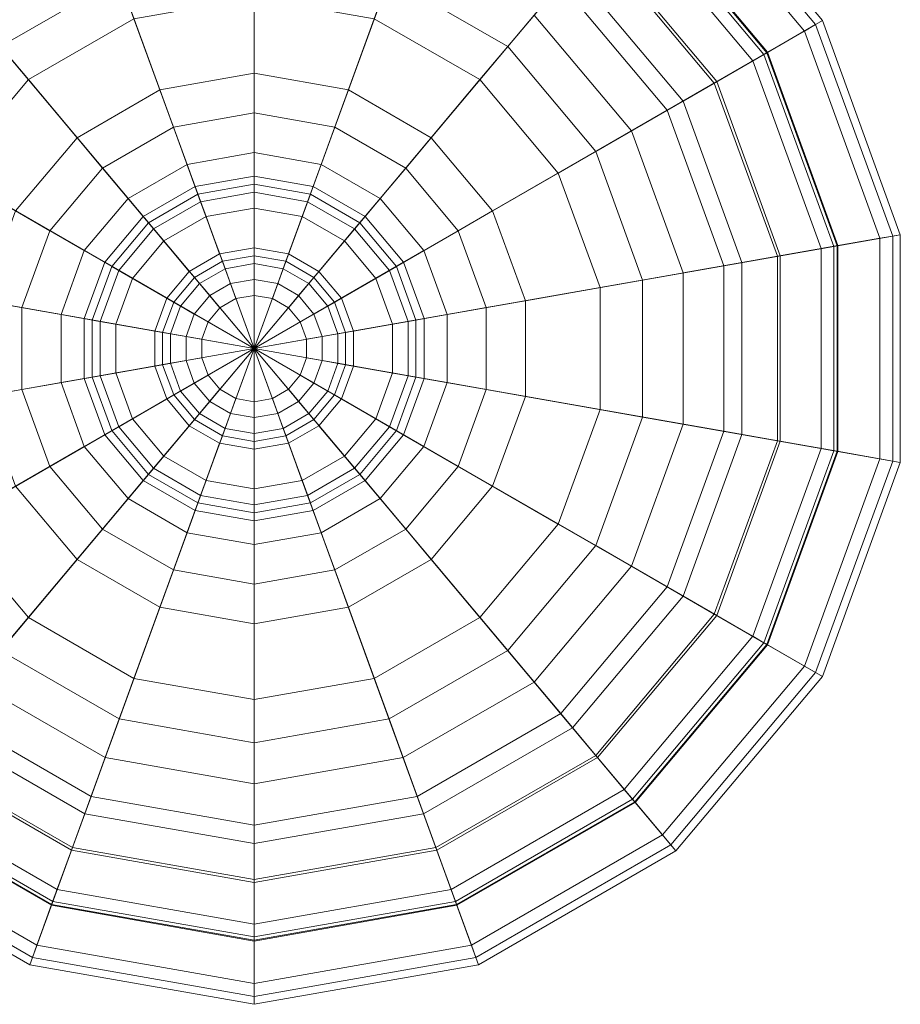
# Model space of a CAD drawing. Units: inches. Extents: x 375 to 1122, y 27 to 1069.
# Tile 14 of 155: x 729.198 to 731.015, y 267.095 to 269.129. Entities that reach past the tile are written whole.
import ezdxf

# ---------------------------------------------------------------- set-up
doc = ezdxf.new("R2010")
doc.units = ezdxf.units.IN
doc.layers.add('Furniture', color=30, linetype='Continuous', lineweight=18)

# ---------------------------------------------------------------- blocks, each defined once
blk = doc.blocks.new('A$C403C54AD')
for points in [[(1.940462, 1.15174, -0.060915), (1.946342, 1.118392, -0.057836), (1.946342, 1.118392, -0.057836), (1.929411, 1.147718, -0.060915)], [(1.941029, 1.148524, -0.057684), (1.940462, 1.15174, -0.060915), (1.929411, 1.147718, -0.060915), (1.931044, 1.144889, -0.057684)], [(1.952223, 1.15174, -0.060915), (1.946342, 1.118392, -0.057836), (1.946342, 1.118392, -0.057836), (1.940462, 1.15174, -0.060915)], [(1.951655, 1.148524, -0.057684), (1.952223, 1.15174, -0.060915), (1.940462, 1.15174, -0.060915), (1.941029, 1.148524, -0.057684)], [(1.963274, 1.147718, -0.060915), (1.946342, 1.118392, -0.057836), (1.946342, 1.118392, -0.057836), (1.952223, 1.15174, -0.060915)], [(1.961641, 1.144889, -0.057684), (1.963274, 1.147718, -0.060915), (1.952223, 1.15174, -0.060915), (1.951655, 1.148524, -0.057684)], [(1.941036, 1.148484, 0.102069), (1.940532, 1.151347, 0.088845), (1.929611, 1.147372, 0.088845), (1.931064, 1.144854, 0.102069)], [(1.940532, 1.151347, 0.088845), (1.940649, 1.150682, 0.060603), (1.929948, 1.146788, 0.060603), (1.929611, 1.147372, 0.088845)], [(1.951648, 1.148484, 0.102069), (1.952153, 1.151347, 0.088845), (1.940532, 1.151347, 0.088845), (1.941036, 1.148484, 0.102069)], [(1.952153, 1.151347, 0.088845), (1.952036, 1.150682, 0.060603), (1.940649, 1.150682, 0.060603), (1.940532, 1.151347, 0.088845)], [(1.96162, 1.144854, 0.102069), (1.963074, 1.147372, 0.088845), (1.952153, 1.151347, 0.088845), (1.951648, 1.148484, 0.102069)], [(1.963074, 1.147372, 0.088845), (1.962737, 1.146788, 0.060603), (1.952036, 1.150682, 0.060603), (1.952153, 1.151347, 0.088845)], [(1.940649, 1.150682, 0.060603), (1.94158, 1.145399, 0.042594), (1.932631, 1.142142, 0.042594), (1.929948, 1.146788, 0.060603)], [(1.952036, 1.150682, 0.060603), (1.951105, 1.145399, 0.042594), (1.94158, 1.145399, 0.042594), (1.940649, 1.150682, 0.060603)], [(1.962737, 1.146788, 0.060603), (1.960054, 1.142142, 0.042594), (1.951105, 1.145399, 0.042594), (1.952036, 1.150682, 0.060603)], [(1.943874, 1.13239, -0.054409), (1.941029, 1.148524, -0.057684), (1.931044, 1.144889, -0.057684), (1.939235, 1.130702, -0.054409)], [(1.941904, 1.143563, 0.111475), (1.941036, 1.148484, 0.102069), (1.931064, 1.144854, 0.102069), (1.933563, 1.140527, 0.111475)], [(1.941067, 1.148309, 0.088628), (1.941555, 1.145542, 0.101264), (1.932558, 1.142268, 0.101264), (1.931153, 1.144701, 0.088628)], [(1.941182, 1.147661, 0.061088), (1.941067, 1.148309, 0.088628), (1.931153, 1.144701, 0.088628), (1.931482, 1.144131, 0.061088)], [(1.948811, 1.13239, -0.054409), (1.951655, 1.148524, -0.057684), (1.941029, 1.148524, -0.057684), (1.943874, 1.13239, -0.054409)], [(1.950781, 1.143563, 0.111475), (1.951648, 1.148484, 0.102069), (1.941036, 1.148484, 0.102069), (1.941904, 1.143563, 0.111475)], [(1.951618, 1.148309, 0.088628), (1.95113, 1.145542, 0.101264), (1.941555, 1.145542, 0.101264), (1.941067, 1.148309, 0.088628)], [(1.951503, 1.147661, 0.061088), (1.951618, 1.148309, 0.088628), (1.941067, 1.148309, 0.088628), (1.941182, 1.147661, 0.061088)], [(1.95345, 1.130702, -0.054409), (1.961641, 1.144889, -0.057684), (1.951655, 1.148524, -0.057684), (1.948811, 1.13239, -0.054409)], [(1.959122, 1.140527, 0.111475), (1.96162, 1.144854, 0.102069), (1.951648, 1.148484, 0.102069), (1.950781, 1.143563, 0.111475)], [(1.961532, 1.144701, 0.088628), (1.960127, 1.142268, 0.101264), (1.95113, 1.145542, 0.101264), (1.951618, 1.148309, 0.088628)], [(1.961203, 1.144131, 0.061088), (1.961532, 1.144701, 0.088628), (1.951618, 1.148309, 0.088628), (1.951503, 1.147661, 0.061088)], [(1.929411, 1.147718, -0.060915), (1.946342, 1.118392, -0.057836), (1.946342, 1.118392, -0.057836), (1.920403, 1.140158, -0.060915)], [(1.931044, 1.144889, -0.057684), (1.929411, 1.147718, -0.060915), (1.920403, 1.140158, -0.060915), (1.922904, 1.138059, -0.057684)], [(1.942068, 1.142631, 0.043942), (1.941182, 1.147661, 0.061088), (1.931482, 1.144131, 0.061088), (1.934036, 1.139708, 0.043942)], [(1.950616, 1.142631, 0.043942), (1.951503, 1.147661, 0.061088), (1.941182, 1.147661, 0.061088), (1.942068, 1.142631, 0.043942)], [(1.972282, 1.140158, -0.060915), (1.946342, 1.118392, -0.057836), (1.946342, 1.118392, -0.057836), (1.963274, 1.147718, -0.060915)], [(1.958649, 1.139708, 0.043942), (1.961203, 1.144131, 0.061088), (1.951503, 1.147661, 0.061088), (1.950616, 1.142631, 0.043942)], [(1.969781, 1.138059, -0.057684), (1.972282, 1.140158, -0.060915), (1.963274, 1.147718, -0.060915), (1.961641, 1.144889, -0.057684)], [(1.931064, 1.144854, 0.102069), (1.929611, 1.147372, 0.088845), (1.920708, 1.139902, 0.088845), (1.922935, 1.138033, 0.102069)], [(1.929611, 1.147372, 0.088845), (1.929948, 1.146788, 0.060603), (1.921225, 1.139468, 0.060603), (1.920708, 1.139902, 0.088845)], [(1.96975, 1.138033, 0.102069), (1.971977, 1.139902, 0.088845), (1.963074, 1.147372, 0.088845), (1.96162, 1.144854, 0.102069)], [(1.971977, 1.139902, 0.088845), (1.97146, 1.139468, 0.060603), (1.962737, 1.146788, 0.060603), (1.963074, 1.147372, 0.088845)], [(1.929948, 1.146788, 0.060603), (1.932631, 1.142142, 0.042594), (1.925335, 1.13602, 0.042594), (1.921225, 1.139468, 0.060603)], [(1.97146, 1.139468, 0.060603), (1.96735, 1.13602, 0.042594), (1.960054, 1.142142, 0.042594), (1.962737, 1.146788, 0.060603)], [(1.941555, 1.145542, 0.101264), (1.942439, 1.140532, 0.111475), (1.935102, 1.137861, 0.111475), (1.932558, 1.142268, 0.101264)], [(1.95113, 1.145542, 0.101264), (1.950246, 1.140532, 0.111475), (1.942439, 1.140532, 0.111475), (1.941555, 1.145542, 0.101264)], [(1.960127, 1.142268, 0.101264), (1.957583, 1.137861, 0.111475), (1.950246, 1.140532, 0.111475), (1.95113, 1.145542, 0.101264)], [(1.94158, 1.145399, 0.042594), (1.942807, 1.13844, 0.032362), (1.936164, 1.136022, 0.032362), (1.932631, 1.142142, 0.042594)], [(1.951105, 1.145399, 0.042594), (1.949878, 1.13844, 0.032362), (1.942807, 1.13844, 0.032362), (1.94158, 1.145399, 0.042594)], [(1.960054, 1.142142, 0.042594), (1.956521, 1.136022, 0.032362), (1.949878, 1.13844, 0.032362), (1.951105, 1.145399, 0.042594)], [(1.939235, 1.130702, -0.054409), (1.931044, 1.144889, -0.057684), (1.922904, 1.138059, -0.057684), (1.935454, 1.127529, -0.054409)], [(1.933563, 1.140527, 0.111475), (1.931064, 1.144854, 0.102069), (1.922935, 1.138033, 0.102069), (1.926763, 1.134821, 0.111475)], [(1.931153, 1.144701, 0.088628), (1.932558, 1.142268, 0.101264), (1.925223, 1.136113, 0.101264), (1.923071, 1.137919, 0.088628)], [(1.931482, 1.144131, 0.061088), (1.931153, 1.144701, 0.088628), (1.923071, 1.137919, 0.088628), (1.923575, 1.137496, 0.061088)], [(1.957231, 1.127529, -0.054409), (1.969781, 1.138059, -0.057684), (1.961641, 1.144889, -0.057684), (1.95345, 1.130702, -0.054409)], [(1.965922, 1.134821, 0.111475), (1.96975, 1.138033, 0.102069), (1.96162, 1.144854, 0.102069), (1.959122, 1.140527, 0.111475)], [(1.969614, 1.137919, 0.088628), (1.967462, 1.136113, 0.101264), (1.960127, 1.142268, 0.101264), (1.961532, 1.144701, 0.088628)], [(1.96911, 1.137496, 0.061088), (1.969614, 1.137919, 0.088628), (1.961532, 1.144701, 0.088628), (1.961203, 1.144131, 0.061088)], [(1.934036, 1.139708, 0.043942), (1.931482, 1.144131, 0.061088), (1.923575, 1.137496, 0.061088), (1.927488, 1.134213, 0.043942)], [(1.965197, 1.134213, 0.043942), (1.96911, 1.137496, 0.061088), (1.961203, 1.144131, 0.061088), (1.958649, 1.139708, 0.043942)], [(1.942439, 1.140532, 0.111475), (1.941904, 1.143563, 0.111475), (1.933563, 1.140527, 0.111475), (1.935102, 1.137861, 0.111475)], [(1.950246, 1.140532, 0.111475), (1.950781, 1.143563, 0.111475), (1.941904, 1.143563, 0.111475), (1.942439, 1.140532, 0.111475)], [(1.957583, 1.137861, 0.111475), (1.959122, 1.140527, 0.111475), (1.950781, 1.143563, 0.111475), (1.950246, 1.140532, 0.111475)], [(1.943195, 1.136244, 0.03455), (1.942068, 1.142631, 0.043942), (1.934036, 1.139708, 0.043942), (1.937279, 1.134091, 0.03455)], [(1.94949, 1.136244, 0.03455), (1.950616, 1.142631, 0.043942), (1.942068, 1.142631, 0.043942), (1.943195, 1.136244, 0.03455)], [(1.955406, 1.134091, 0.03455), (1.958649, 1.139708, 0.043942), (1.950616, 1.142631, 0.043942), (1.94949, 1.136244, 0.03455)], [(1.932558, 1.142268, 0.101264), (1.935102, 1.137861, 0.111475), (1.929121, 1.132843, 0.111475), (1.925223, 1.136113, 0.101264)], [(1.932631, 1.142142, 0.042594), (1.936164, 1.136022, 0.032362), (1.930748, 1.131478, 0.032362), (1.925335, 1.13602, 0.042594)], [(1.96735, 1.13602, 0.042594), (1.961937, 1.131478, 0.032362), (1.956521, 1.136022, 0.032362), (1.960054, 1.142142, 0.042594)], [(1.967462, 1.136113, 0.101264), (1.963564, 1.132843, 0.111475), (1.957583, 1.137861, 0.111475), (1.960127, 1.142268, 0.101264)], [(1.935102, 1.137861, 0.111475), (1.933563, 1.140527, 0.111475), (1.926763, 1.134821, 0.111475), (1.929121, 1.132843, 0.111475)], [(1.963564, 1.132843, 0.111475), (1.965922, 1.134821, 0.111475), (1.959122, 1.140527, 0.111475), (1.957583, 1.137861, 0.111475)], [(1.920403, 1.140158, -0.060915), (1.946342, 1.118392, -0.057836), (1.946342, 1.118392, -0.057836), (1.914522, 1.129974, -0.060915)], [(1.978163, 1.129974, -0.060915), (1.946342, 1.118392, -0.057836), (1.946342, 1.118392, -0.057836), (1.972282, 1.140158, -0.060915)], [(1.975094, 1.128857, -0.057684), (1.978163, 1.129974, -0.060915), (1.972282, 1.140158, -0.060915), (1.969781, 1.138059, -0.057684)], [(1.937279, 1.134091, 0.03455), (1.934036, 1.139708, 0.043942), (1.927488, 1.134213, 0.043942), (1.932456, 1.130044, 0.03455)], [(1.960229, 1.130044, 0.03455), (1.965197, 1.134213, 0.043942), (1.958649, 1.139708, 0.043942), (1.955406, 1.134091, 0.03455)], [(1.977153, 1.129606, 0.060603), (1.972112, 1.127772, 0.042594), (1.96735, 1.13602, 0.042594), (1.97146, 1.139468, 0.060603)], [(1.975056, 1.128843, 0.102069), (1.977788, 1.129837, 0.088845), (1.971977, 1.139902, 0.088845), (1.96975, 1.138033, 0.102069)], [(1.977788, 1.129837, 0.088845), (1.977153, 1.129606, 0.060603), (1.97146, 1.139468, 0.060603), (1.971977, 1.139902, 0.088845)], [(1.942807, 1.13844, 0.032362), (1.944585, 1.128357, 0.024995), (1.941283, 1.127155, 0.024995), (1.936164, 1.136022, 0.032362)], [(1.949878, 1.13844, 0.032362), (1.9481, 1.128357, 0.024995), (1.944585, 1.128357, 0.024995), (1.942807, 1.13844, 0.032362)], [(1.956521, 1.136022, 0.032362), (1.951402, 1.127155, 0.024995), (1.9481, 1.128357, 0.024995), (1.949878, 1.13844, 0.032362)], [(1.935454, 1.127529, -0.054409), (1.922904, 1.138059, -0.057684), (1.917591, 1.128857, -0.057684), (1.932985, 1.123254, -0.054409)], [(1.9597, 1.123254, -0.054409), (1.975094, 1.128857, -0.057684), (1.969781, 1.138059, -0.057684), (1.957231, 1.127529, -0.054409)], [(1.970361, 1.127134, 0.111475), (1.975056, 1.128843, 0.102069), (1.96975, 1.138033, 0.102069), (1.965922, 1.134821, 0.111475)], [(1.974889, 1.128782, 0.088628), (1.972249, 1.127821, 0.101264), (1.967462, 1.136113, 0.101264), (1.969614, 1.137919, 0.088628)], [(1.974271, 1.128557, 0.061088), (1.974889, 1.128782, 0.088628), (1.969614, 1.137919, 0.088628), (1.96911, 1.137496, 0.061088)], [(1.969471, 1.12681, 0.043942), (1.974271, 1.128557, 0.061088), (1.96911, 1.137496, 0.061088), (1.965197, 1.134213, 0.043942)], [(1.925335, 1.13602, 0.042594), (1.930748, 1.131478, 0.032362), (1.927213, 1.125355, 0.032362), (1.920572, 1.127772, 0.042594)], [(1.936164, 1.136022, 0.032362), (1.941283, 1.127155, 0.024995), (1.938591, 1.124896, 0.024995), (1.930748, 1.131478, 0.032362)], [(1.944796, 1.127161, 0.027913), (1.943195, 1.136244, 0.03455), (1.937279, 1.134091, 0.03455), (1.94189, 1.126103, 0.027913)], [(1.947889, 1.127161, 0.027913), (1.94949, 1.136244, 0.03455), (1.943195, 1.136244, 0.03455), (1.944796, 1.127161, 0.027913)], [(1.950795, 1.126103, 0.027913), (1.955406, 1.134091, 0.03455), (1.94949, 1.136244, 0.03455), (1.947889, 1.127161, 0.027913)], [(1.961937, 1.131478, 0.032362), (1.954094, 1.124896, 0.024995), (1.951402, 1.127155, 0.024995), (1.956521, 1.136022, 0.032362)], [(1.972112, 1.127772, 0.042594), (1.965472, 1.125355, 0.032362), (1.961937, 1.131478, 0.032362), (1.96735, 1.13602, 0.042594)], [(1.972249, 1.127821, 0.101264), (1.967468, 1.126081, 0.111475), (1.963564, 1.132843, 0.111475), (1.967462, 1.136113, 0.101264)], [(1.967468, 1.126081, 0.111475), (1.970361, 1.127134, 0.111475), (1.965922, 1.134821, 0.111475), (1.963564, 1.132843, 0.111475)], [(1.932456, 1.130044, 0.03455), (1.927488, 1.134213, 0.043942), (1.923214, 1.12681, 0.043942), (1.929308, 1.124592, 0.03455)], [(1.94189, 1.126103, 0.027913), (1.937279, 1.134091, 0.03455), (1.932456, 1.130044, 0.03455), (1.939522, 1.124116, 0.027913)], [(1.953163, 1.124116, 0.027913), (1.960229, 1.130044, 0.03455), (1.955406, 1.134091, 0.03455), (1.950795, 1.126103, 0.027913)], [(1.963376, 1.124592, 0.03455), (1.969471, 1.12681, 0.043942), (1.965197, 1.134213, 0.043942), (1.960229, 1.130044, 0.03455)], [(1.94423, 1.130374, -0.051544), (1.943874, 1.13239, -0.054409), (1.939235, 1.130702, -0.054409), (1.940259, 1.128929, -0.051544)], [(1.948455, 1.130374, -0.051544), (1.948811, 1.13239, -0.054409), (1.943874, 1.13239, -0.054409), (1.94423, 1.130374, -0.051544)], [(1.952426, 1.128929, -0.051544), (1.95345, 1.130702, -0.054409), (1.948811, 1.13239, -0.054409), (1.948455, 1.130374, -0.051544)], [(1.930748, 1.131478, 0.032362), (1.938591, 1.124896, 0.024995), (1.936834, 1.121853, 0.024995), (1.927213, 1.125355, 0.032362)], [(1.965472, 1.125355, 0.032362), (1.955851, 1.121853, 0.024995), (1.954094, 1.124896, 0.024995), (1.961937, 1.131478, 0.032362)], [(1.940259, 1.128929, -0.051544), (1.939235, 1.130702, -0.054409), (1.935454, 1.127529, -0.054409), (1.937022, 1.126213, -0.051544)], [(1.944941, 1.12634, -0.049498), (1.94423, 1.130374, -0.051544), (1.940259, 1.128929, -0.051544), (1.942307, 1.125382, -0.049498)], [(1.947744, 1.12634, -0.049498), (1.948455, 1.130374, -0.051544), (1.94423, 1.130374, -0.051544), (1.944941, 1.12634, -0.049498)], [(1.950378, 1.125382, -0.049498), (1.952426, 1.128929, -0.051544), (1.948455, 1.130374, -0.051544), (1.947744, 1.12634, -0.049498)], [(1.955663, 1.126213, -0.051544), (1.957231, 1.127529, -0.054409), (1.95345, 1.130702, -0.054409), (1.952426, 1.128929, -0.051544)], [(1.914522, 1.129974, -0.060915), (1.946342, 1.118392, -0.057836), (1.946342, 1.118392, -0.057836), (1.91248, 1.118392, -0.060915)], [(1.939522, 1.124116, 0.027913), (1.932456, 1.130044, 0.03455), (1.929308, 1.124592, 0.03455), (1.937975, 1.121437, 0.027913)], [(1.980205, 1.118392, -0.060915), (1.946342, 1.118392, -0.057836), (1.946342, 1.118392, -0.057836), (1.978163, 1.129974, -0.060915)], [(1.95471, 1.121437, 0.027913), (1.963376, 1.124592, 0.03455), (1.960229, 1.130044, 0.03455), (1.953163, 1.124116, 0.027913)], [(1.976898, 1.118392, 0.102069), (1.979806, 1.118392, 0.088845), (1.977788, 1.129837, 0.088845), (1.975056, 1.128843, 0.102069)], [(1.976939, 1.118392, -0.057684), (1.980205, 1.118392, -0.060915), (1.978163, 1.129974, -0.060915), (1.975094, 1.128857, -0.057684)], [(1.979806, 1.118392, 0.088845), (1.979131, 1.118392, 0.060603), (1.977153, 1.129606, 0.060603), (1.977788, 1.129837, 0.088845)], [(1.979131, 1.118392, 0.060603), (1.973766, 1.118392, 0.042594), (1.972112, 1.127772, 0.042594), (1.977153, 1.129606, 0.060603)], [(1.932985, 1.123254, -0.054409), (1.917591, 1.128857, -0.057684), (1.915746, 1.118392, -0.057684), (1.932128, 1.118392, -0.054409)], [(1.942307, 1.125382, -0.049498), (1.940259, 1.128929, -0.051544), (1.937022, 1.126213, -0.051544), (1.94016, 1.12358, -0.049498)], [(1.952525, 1.12358, -0.049498), (1.955663, 1.126213, -0.051544), (1.952426, 1.128929, -0.051544), (1.950378, 1.125382, -0.049498)], [(1.960557, 1.118392, -0.054409), (1.976939, 1.118392, -0.057684), (1.975094, 1.128857, -0.057684), (1.9597, 1.123254, -0.054409)], [(1.971902, 1.118392, 0.111475), (1.976898, 1.118392, 0.102069), (1.975056, 1.128843, 0.102069), (1.970361, 1.127134, 0.111475)], [(1.976721, 1.118392, 0.088628), (1.973912, 1.118392, 0.101264), (1.972249, 1.127821, 0.101264), (1.974889, 1.128782, 0.088628)], [(1.976063, 1.118392, 0.061088), (1.976721, 1.118392, 0.088628), (1.974889, 1.128782, 0.088628), (1.974271, 1.128557, 0.061088)], [(1.944585, 1.128357, 0.024995), (1.945439, 1.123517, 0.024176), (1.94374, 1.122899, 0.024176), (1.941283, 1.127155, 0.024995)], [(1.9481, 1.128357, 0.024995), (1.947246, 1.123517, 0.024176), (1.945439, 1.123517, 0.024176), (1.944585, 1.128357, 0.024995)], [(1.951402, 1.127155, 0.024995), (1.948945, 1.122899, 0.024176), (1.947246, 1.123517, 0.024176), (1.9481, 1.128357, 0.024995)], [(1.970956, 1.118392, 0.043942), (1.976063, 1.118392, 0.061088), (1.974271, 1.128557, 0.061088), (1.969471, 1.12681, 0.043942)], [(1.973766, 1.118392, 0.042594), (1.9667, 1.118392, 0.032362), (1.965472, 1.125355, 0.032362), (1.972112, 1.127772, 0.042594)], [(1.973912, 1.118392, 0.101264), (1.968824, 1.118392, 0.111475), (1.967468, 1.126081, 0.111475), (1.972249, 1.127821, 0.101264)], [(1.937022, 1.126213, -0.051544), (1.935454, 1.127529, -0.054409), (1.932985, 1.123254, -0.054409), (1.93491, 1.122553, -0.051544)], [(1.957775, 1.122553, -0.051544), (1.9597, 1.123254, -0.054409), (1.957231, 1.127529, -0.054409), (1.955663, 1.126213, -0.051544)], [(1.941283, 1.127155, 0.024995), (1.94374, 1.122899, 0.024176), (1.942356, 1.121737, 0.024176), (1.938591, 1.124896, 0.024995)], [(1.946342, 1.118392, 0.02643), (1.944796, 1.127161, 0.027913), (1.94189, 1.126103, 0.027913), (1.946342, 1.118392, 0.02643)], [(1.94487, 1.126744, 0.021311), (1.945581, 1.122711, 0.019264), (1.94415, 1.12219, 0.019264), (1.942102, 1.125736, 0.021311)], [(1.945083, 1.125534, 0.023357), (1.94487, 1.126744, 0.021311), (1.942102, 1.125736, 0.021311), (1.942717, 1.124672, 0.023357)], [(1.946342, 1.118392, 0.02643), (1.947889, 1.127161, 0.027913), (1.944796, 1.127161, 0.027913), (1.946342, 1.118392, 0.02643)], [(1.947815, 1.126744, 0.021311), (1.947104, 1.122711, 0.019264), (1.945581, 1.122711, 0.019264), (1.94487, 1.126744, 0.021311)], [(1.947602, 1.125534, 0.023357), (1.947815, 1.126744, 0.021311), (1.94487, 1.126744, 0.021311), (1.945083, 1.125534, 0.023357)], [(1.946342, 1.118392, 0.02643), (1.950795, 1.126103, 0.027913), (1.947889, 1.127161, 0.027913), (1.946342, 1.118392, 0.02643)], [(1.950583, 1.125736, 0.021311), (1.948535, 1.12219, 0.019264), (1.947104, 1.122711, 0.019264), (1.947815, 1.126744, 0.021311)], [(1.949968, 1.124672, 0.023357), (1.950583, 1.125736, 0.021311), (1.947815, 1.126744, 0.021311), (1.947602, 1.125534, 0.023357)], [(1.954094, 1.124896, 0.024995), (1.950329, 1.121737, 0.024176), (1.948945, 1.122899, 0.024176), (1.951402, 1.127155, 0.024995)], [(1.96447, 1.118392, 0.03455), (1.970956, 1.118392, 0.043942), (1.969471, 1.12681, 0.043942), (1.963376, 1.124592, 0.03455)], [(1.968824, 1.118392, 0.111475), (1.971902, 1.118392, 0.111475), (1.970361, 1.127134, 0.111475), (1.967468, 1.126081, 0.111475)], [(1.94016, 1.12358, -0.049498), (1.937022, 1.126213, -0.051544), (1.93491, 1.122553, -0.051544), (1.938758, 1.121153, -0.049498)], [(1.94551, 1.123114, -0.044177), (1.944941, 1.12634, -0.049498), (1.942307, 1.125382, -0.049498), (1.943945, 1.122544, -0.044177)], [(1.947175, 1.123114, -0.044177), (1.947744, 1.12634, -0.049498), (1.944941, 1.12634, -0.049498), (1.94551, 1.123114, -0.044177)], [(1.94874, 1.122544, -0.044177), (1.950378, 1.125382, -0.049498), (1.947744, 1.12634, -0.049498), (1.947175, 1.123114, -0.044177)], [(1.953927, 1.121153, -0.049498), (1.957775, 1.122553, -0.051544), (1.955663, 1.126213, -0.051544), (1.952525, 1.12358, -0.049498)], [(1.946342, 1.118392, 0.02643), (1.94189, 1.126103, 0.027913), (1.939522, 1.124116, 0.027913), (1.946342, 1.118392, 0.02643)], [(1.942102, 1.125736, 0.021311), (1.94415, 1.12219, 0.019264), (1.942983, 1.121211, 0.019264), (1.939846, 1.123843, 0.021311)], [(1.942717, 1.124672, 0.023357), (1.942102, 1.125736, 0.021311), (1.939846, 1.123843, 0.021311), (1.940787, 1.123054, 0.023357)], [(1.946342, 1.118392, 0.02643), (1.953163, 1.124116, 0.027913), (1.950795, 1.126103, 0.027913), (1.946342, 1.118392, 0.02643)], [(1.952839, 1.123843, 0.021311), (1.949702, 1.121211, 0.019264), (1.948535, 1.12219, 0.019264), (1.950583, 1.125736, 0.021311)], [(1.951898, 1.123054, 0.023357), (1.952839, 1.123843, 0.021311), (1.950583, 1.125736, 0.021311), (1.949968, 1.124672, 0.023357)], [(1.927213, 1.125355, 0.032362), (1.936834, 1.121853, 0.024995), (1.936224, 1.118392, 0.024995), (1.925985, 1.118392, 0.032362)], [(1.943945, 1.122544, -0.044177), (1.942307, 1.125382, -0.049498), (1.94016, 1.12358, -0.049498), (1.94267, 1.121474, -0.044177)], [(1.945439, 1.123517, 0.024176), (1.945083, 1.125534, 0.023357), (1.942717, 1.124672, 0.023357), (1.94374, 1.122899, 0.024176)], [(1.947246, 1.123517, 0.024176), (1.947602, 1.125534, 0.023357), (1.945083, 1.125534, 0.023357), (1.945439, 1.123517, 0.024176)], [(1.948945, 1.122899, 0.024176), (1.949968, 1.124672, 0.023357), (1.947602, 1.125534, 0.023357), (1.947246, 1.123517, 0.024176)], [(1.950015, 1.121474, -0.044177), (1.952525, 1.12358, -0.049498), (1.950378, 1.125382, -0.049498), (1.94874, 1.122544, -0.044177)], [(1.9667, 1.118392, 0.032362), (1.956461, 1.118392, 0.024995), (1.955851, 1.121853, 0.024995), (1.965472, 1.125355, 0.032362)], [(1.938591, 1.124896, 0.024995), (1.942356, 1.121737, 0.024176), (1.941452, 1.120172, 0.024176), (1.936834, 1.121853, 0.024995)], [(1.955851, 1.121853, 0.024995), (1.951233, 1.120172, 0.024176), (1.950329, 1.121737, 0.024176), (1.954094, 1.124896, 0.024995)], [(1.937975, 1.121437, 0.027913), (1.929308, 1.124592, 0.03455), (1.928215, 1.118392, 0.03455), (1.937438, 1.118392, 0.027913)], [(1.94374, 1.122899, 0.024176), (1.942717, 1.124672, 0.023357), (1.940787, 1.123054, 0.023357), (1.942356, 1.121737, 0.024176)], [(1.950329, 1.121737, 0.024176), (1.951898, 1.123054, 0.023357), (1.949968, 1.124672, 0.023357), (1.948945, 1.122899, 0.024176)], [(1.955247, 1.118392, 0.027913), (1.96447, 1.118392, 0.03455), (1.963376, 1.124592, 0.03455), (1.95471, 1.121437, 0.027913)], [(1.946342, 1.118392, 0.02643), (1.939522, 1.124116, 0.027913), (1.937975, 1.121437, 0.027913), (1.946342, 1.118392, 0.02643)], [(1.939846, 1.123843, 0.021311), (1.942983, 1.121211, 0.019264), (1.942222, 1.119892, 0.019264), (1.938373, 1.121293, 0.021311)], [(1.940787, 1.123054, 0.023357), (1.939846, 1.123843, 0.021311), (1.938373, 1.121293, 0.021311), (1.939528, 1.120872, 0.023357)], [(1.946342, 1.118392, 0.02643), (1.95471, 1.121437, 0.027913), (1.953163, 1.124116, 0.027913), (1.946342, 1.118392, 0.02643)], [(1.954312, 1.121293, 0.021311), (1.950463, 1.119892, 0.019264), (1.949702, 1.121211, 0.019264), (1.952839, 1.123843, 0.021311)], [(1.953157, 1.120872, 0.023357), (1.954312, 1.121293, 0.021311), (1.952839, 1.123843, 0.021311), (1.951898, 1.123054, 0.023357)], [(1.93491, 1.122553, -0.051544), (1.932985, 1.123254, -0.054409), (1.932128, 1.118392, -0.054409), (1.934176, 1.118392, -0.051544)], [(1.94267, 1.121474, -0.044177), (1.94016, 1.12358, -0.049498), (1.938758, 1.121153, -0.049498), (1.941837, 1.120032, -0.044177)], [(1.950848, 1.120032, -0.044177), (1.953927, 1.121153, -0.049498), (1.952525, 1.12358, -0.049498), (1.950015, 1.121474, -0.044177)], [(1.958509, 1.118392, -0.051544), (1.960557, 1.118392, -0.054409), (1.9597, 1.123254, -0.054409), (1.957775, 1.122553, -0.051544)], [(1.942356, 1.121737, 0.024176), (1.940787, 1.123054, 0.023357), (1.939528, 1.120872, 0.023357), (1.941452, 1.120172, 0.024176)], [(1.945723, 1.121904, -0.035582), (1.94551, 1.123114, -0.044177), (1.943945, 1.122544, -0.044177), (1.94456, 1.12148, -0.035582)], [(1.945581, 1.122711, 0.019264), (1.945865, 1.121097, 0.012716), (1.944969, 1.120771, 0.012716), (1.94415, 1.12219, 0.019264)], [(1.946962, 1.121904, -0.035582), (1.947175, 1.123114, -0.044177), (1.94551, 1.123114, -0.044177), (1.945723, 1.121904, -0.035582)], [(1.947104, 1.122711, 0.019264), (1.946819, 1.121097, 0.012716), (1.945865, 1.121097, 0.012716), (1.945581, 1.122711, 0.019264)], [(1.948535, 1.12219, 0.019264), (1.947716, 1.120771, 0.012716), (1.946819, 1.121097, 0.012716), (1.947104, 1.122711, 0.019264)], [(1.948125, 1.12148, -0.035582), (1.94874, 1.122544, -0.044177), (1.947175, 1.123114, -0.044177), (1.946962, 1.121904, -0.035582)], [(1.951233, 1.120172, 0.024176), (1.953157, 1.120872, 0.023357), (1.951898, 1.123054, 0.023357), (1.950329, 1.121737, 0.024176)], [(1.938758, 1.121153, -0.049498), (1.93491, 1.122553, -0.051544), (1.934176, 1.118392, -0.051544), (1.938271, 1.118392, -0.049498)], [(1.94456, 1.12148, -0.035582), (1.943945, 1.122544, -0.044177), (1.94267, 1.121474, -0.044177), (1.943611, 1.120684, -0.035582)], [(1.94415, 1.12219, 0.019264), (1.944969, 1.120771, 0.012716), (1.944238, 1.120158, 0.012716), (1.942983, 1.121211, 0.019264)], [(1.949702, 1.121211, 0.019264), (1.948447, 1.120158, 0.012716), (1.947716, 1.120771, 0.012716), (1.948535, 1.12219, 0.019264)], [(1.949074, 1.120684, -0.035582), (1.950015, 1.121474, -0.044177), (1.94874, 1.122544, -0.044177), (1.948125, 1.12148, -0.035582)], [(1.954413, 1.118392, -0.049498), (1.958509, 1.118392, -0.051544), (1.957775, 1.122553, -0.051544), (1.953927, 1.121153, -0.049498)], [(1.936834, 1.121853, 0.024995), (1.941452, 1.120172, 0.024176), (1.941138, 1.118392, 0.024176), (1.936224, 1.118392, 0.024995)], [(1.945865, 1.121097, 0.012716), (1.945723, 1.121904, -0.035582), (1.94456, 1.12148, -0.035582), (1.944969, 1.120771, 0.012716)], [(1.946819, 1.121097, 0.012716), (1.946962, 1.121904, -0.035582), (1.945723, 1.121904, -0.035582), (1.945865, 1.121097, 0.012716)], [(1.947716, 1.120771, 0.012716), (1.948125, 1.12148, -0.035582), (1.946962, 1.121904, -0.035582), (1.946819, 1.121097, 0.012716)], [(1.956461, 1.118392, 0.024995), (1.951547, 1.118392, 0.024176), (1.951233, 1.120172, 0.024176), (1.955851, 1.121853, 0.024995)], [(1.946342, 1.118392, 0.02643), (1.937975, 1.121437, 0.027913), (1.937438, 1.118392, 0.027913), (1.946342, 1.118392, 0.02643)], [(1.938373, 1.121293, 0.021311), (1.942222, 1.119892, 0.019264), (1.941957, 1.118392, 0.019264), (1.937862, 1.118392, 0.021311)], [(1.939528, 1.120872, 0.023357), (1.938373, 1.121293, 0.021311), (1.937862, 1.118392, 0.021311), (1.939091, 1.118392, 0.023357)], [(1.941837, 1.120032, -0.044177), (1.938758, 1.121153, -0.049498), (1.938271, 1.118392, -0.049498), (1.941548, 1.118392, -0.044177)], [(1.943611, 1.120684, -0.035582), (1.94267, 1.121474, -0.044177), (1.941837, 1.120032, -0.044177), (1.942992, 1.119612, -0.035582)], [(1.942983, 1.121211, 0.019264), (1.944238, 1.120158, 0.012716), (1.943761, 1.119332, 0.012716), (1.942222, 1.119892, 0.019264)], [(1.944969, 1.120771, 0.012716), (1.94456, 1.12148, -0.035582), (1.943611, 1.120684, -0.035582), (1.944238, 1.120158, 0.012716)], [(1.946342, 1.118392, 0.02643), (1.955247, 1.118392, 0.027913), (1.95471, 1.121437, 0.027913), (1.946342, 1.118392, 0.02643)], [(1.948447, 1.120158, 0.012716), (1.949074, 1.120684, -0.035582), (1.948125, 1.12148, -0.035582), (1.947716, 1.120771, 0.012716)], [(1.950463, 1.119892, 0.019264), (1.948924, 1.119332, 0.012716), (1.948447, 1.120158, 0.012716), (1.949702, 1.121211, 0.019264)], [(1.949693, 1.119612, -0.035582), (1.950848, 1.120032, -0.044177), (1.950015, 1.121474, -0.044177), (1.949074, 1.120684, -0.035582)], [(1.954823, 1.118392, 0.021311), (1.950727, 1.118392, 0.019264), (1.950463, 1.119892, 0.019264), (1.954312, 1.121293, 0.021311)], [(1.951137, 1.118392, -0.044177), (1.954413, 1.118392, -0.049498), (1.953927, 1.121153, -0.049498), (1.950848, 1.120032, -0.044177)], [(1.953594, 1.118392, 0.023357), (1.954823, 1.118392, 0.021311), (1.954312, 1.121293, 0.021311), (1.953157, 1.120872, 0.023357)], [(1.941452, 1.120172, 0.024176), (1.939528, 1.120872, 0.023357), (1.939091, 1.118392, 0.023357), (1.941138, 1.118392, 0.024176)], [(1.944238, 1.120158, 0.012716), (1.943611, 1.120684, -0.035582), (1.942992, 1.119612, -0.035582), (1.943761, 1.119332, 0.012716)], [(1.948924, 1.119332, 0.012716), (1.949693, 1.119612, -0.035582), (1.949074, 1.120684, -0.035582), (1.948447, 1.120158, 0.012716)], [(1.951547, 1.118392, 0.024176), (1.953594, 1.118392, 0.023357), (1.953157, 1.120872, 0.023357), (1.951233, 1.120172, 0.024176)], [(1.942992, 1.119612, -0.035582), (1.941837, 1.120032, -0.044177), (1.941548, 1.118392, -0.044177), (1.942777, 1.118392, -0.035582)], [(1.942222, 1.119892, 0.019264), (1.943761, 1.119332, 0.012716), (1.943596, 1.118392, 0.012716), (1.941957, 1.118392, 0.019264)], [(1.943761, 1.119332, 0.012716), (1.942992, 1.119612, -0.035582), (1.942777, 1.118392, -0.035582), (1.943596, 1.118392, 0.012716)], [(1.950727, 1.118392, 0.019264), (1.949089, 1.118392, 0.012716), (1.948924, 1.119332, 0.012716), (1.950463, 1.119892, 0.019264)], [(1.949089, 1.118392, 0.012716), (1.949908, 1.118392, -0.035582), (1.949693, 1.119612, -0.035582), (1.948924, 1.119332, 0.012716)], [(1.949908, 1.118392, -0.035582), (1.951137, 1.118392, -0.044177), (1.950848, 1.120032, -0.044177), (1.949693, 1.119612, -0.035582)], [(1.91248, 1.118392, -0.060915), (1.946342, 1.118392, -0.057836), (1.946342, 1.118392, -0.057836), (1.914522, 1.106811, -0.060915)], [(1.914522, 1.106811, -0.060915), (1.946342, 1.118392, -0.057836), (1.946342, 1.118392, -0.057836), (1.920403, 1.096626, -0.060915)], [(1.932128, 1.118392, -0.054409), (1.915746, 1.118392, -0.057684), (1.917591, 1.107928, -0.057684), (1.932985, 1.113531, -0.054409)], [(1.920403, 1.096626, -0.060915), (1.946342, 1.118392, -0.057836), (1.946342, 1.118392, -0.057836), (1.929411, 1.089067, -0.060915)], [(1.925985, 1.118392, 0.032362), (1.936224, 1.118392, 0.024995), (1.936834, 1.114931, 0.024995), (1.927213, 1.111429, 0.032362)], [(1.937438, 1.118392, 0.027913), (1.928215, 1.118392, 0.03455), (1.929308, 1.112192, 0.03455), (1.937975, 1.115347, 0.027913)], [(1.929411, 1.089067, -0.060915), (1.946342, 1.118392, -0.057836), (1.946342, 1.118392, -0.057836), (1.940462, 1.085044, -0.060915)], [(1.934176, 1.118392, -0.051544), (1.932128, 1.118392, -0.054409), (1.932985, 1.113531, -0.054409), (1.93491, 1.114231, -0.051544)], [(1.938271, 1.118392, -0.049498), (1.934176, 1.118392, -0.051544), (1.93491, 1.114231, -0.051544), (1.938758, 1.115632, -0.049498)], [(1.936224, 1.118392, 0.024995), (1.941138, 1.118392, 0.024176), (1.941452, 1.116612, 0.024176), (1.936834, 1.114931, 0.024995)], [(1.946342, 1.118392, 0.02643), (1.937438, 1.118392, 0.027913), (1.937975, 1.115347, 0.027913), (1.946342, 1.118392, 0.02643)], [(1.937862, 1.118392, 0.021311), (1.941957, 1.118392, 0.019264), (1.942222, 1.116892, 0.019264), (1.938373, 1.115492, 0.021311)], [(1.939091, 1.118392, 0.023357), (1.937862, 1.118392, 0.021311), (1.938373, 1.115492, 0.021311), (1.939528, 1.115912, 0.023357)], [(1.946342, 1.118392, 0.02643), (1.937975, 1.115347, 0.027913), (1.939522, 1.112669, 0.027913), (1.946342, 1.118392, 0.02643)], [(1.941548, 1.118392, -0.044177), (1.938271, 1.118392, -0.049498), (1.938758, 1.115632, -0.049498), (1.941837, 1.116752, -0.044177)], [(1.941138, 1.118392, 0.024176), (1.939091, 1.118392, 0.023357), (1.939528, 1.115912, 0.023357), (1.941452, 1.116612, 0.024176)], [(1.946342, 1.118392, 0.02643), (1.939522, 1.112669, 0.027913), (1.94189, 1.110681, 0.027913), (1.946342, 1.118392, 0.02643)], [(1.940462, 1.085044, -0.060915), (1.946342, 1.118392, -0.057836), (1.946342, 1.118392, -0.057836), (1.952223, 1.085044, -0.060915)], [(1.942777, 1.118392, -0.035582), (1.941548, 1.118392, -0.044177), (1.941837, 1.116752, -0.044177), (1.942992, 1.117172, -0.035582)], [(1.946342, 1.118392, 0.02643), (1.94189, 1.110681, 0.027913), (1.944796, 1.109623, 0.027913), (1.946342, 1.118392, 0.02643)], [(1.941957, 1.118392, 0.019264), (1.943596, 1.118392, 0.012716), (1.943761, 1.117453, 0.012716), (1.942222, 1.116892, 0.019264)], [(1.943596, 1.118392, 0.012716), (1.942777, 1.118392, -0.035582), (1.942992, 1.117172, -0.035582), (1.943761, 1.117453, 0.012716)], [(1.946342, 1.118392, 0.02643), (1.944796, 1.109623, 0.027913), (1.947889, 1.109623, 0.027913), (1.946342, 1.118392, 0.02643)], [(1.946342, 1.118392, 0.02643), (1.95471, 1.115347, 0.027913), (1.955247, 1.118392, 0.027913), (1.946342, 1.118392, 0.02643)], [(1.946342, 1.118392, 0.02643), (1.953163, 1.112669, 0.027913), (1.95471, 1.115347, 0.027913), (1.946342, 1.118392, 0.02643)], [(1.946342, 1.118392, 0.02643), (1.950795, 1.110681, 0.027913), (1.953163, 1.112669, 0.027913), (1.946342, 1.118392, 0.02643)], [(1.946342, 1.118392, 0.02643), (1.947889, 1.109623, 0.027913), (1.950795, 1.110681, 0.027913), (1.946342, 1.118392, 0.02643)], [(1.972282, 1.096626, -0.060915), (1.946342, 1.118392, -0.057836), (1.946342, 1.118392, -0.057836), (1.978163, 1.106811, -0.060915)], [(1.963274, 1.089067, -0.060915), (1.946342, 1.118392, -0.057836), (1.946342, 1.118392, -0.057836), (1.972282, 1.096626, -0.060915)], [(1.952223, 1.085044, -0.060915), (1.946342, 1.118392, -0.057836), (1.946342, 1.118392, -0.057836), (1.963274, 1.089067, -0.060915)], [(1.978163, 1.106811, -0.060915), (1.946342, 1.118392, -0.057836), (1.946342, 1.118392, -0.057836), (1.980205, 1.118392, -0.060915)], [(1.950463, 1.116892, 0.019264), (1.948924, 1.117453, 0.012716), (1.949089, 1.118392, 0.012716), (1.950727, 1.118392, 0.019264)], [(1.948924, 1.117453, 0.012716), (1.949693, 1.117172, -0.035582), (1.949908, 1.118392, -0.035582), (1.949089, 1.118392, 0.012716)], [(1.949693, 1.117172, -0.035582), (1.950848, 1.116752, -0.044177), (1.951137, 1.118392, -0.044177), (1.949908, 1.118392, -0.035582)], [(1.954312, 1.115492, 0.021311), (1.950463, 1.116892, 0.019264), (1.950727, 1.118392, 0.019264), (1.954823, 1.118392, 0.021311)], [(1.950848, 1.116752, -0.044177), (1.953927, 1.115632, -0.049498), (1.954413, 1.118392, -0.049498), (1.951137, 1.118392, -0.044177)], [(1.951233, 1.116612, 0.024176), (1.953157, 1.115912, 0.023357), (1.953594, 1.118392, 0.023357), (1.951547, 1.118392, 0.024176)], [(1.955851, 1.114931, 0.024995), (1.951233, 1.116612, 0.024176), (1.951547, 1.118392, 0.024176), (1.956461, 1.118392, 0.024995)], [(1.953157, 1.115912, 0.023357), (1.954312, 1.115492, 0.021311), (1.954823, 1.118392, 0.021311), (1.953594, 1.118392, 0.023357)], [(1.953927, 1.115632, -0.049498), (1.957775, 1.114231, -0.051544), (1.958509, 1.118392, -0.051544), (1.954413, 1.118392, -0.049498)], [(1.95471, 1.115347, 0.027913), (1.963376, 1.112192, 0.03455), (1.96447, 1.118392, 0.03455), (1.955247, 1.118392, 0.027913)], [(1.965472, 1.111429, 0.032362), (1.955851, 1.114931, 0.024995), (1.956461, 1.118392, 0.024995), (1.9667, 1.118392, 0.032362)], [(1.957775, 1.114231, -0.051544), (1.9597, 1.113531, -0.054409), (1.960557, 1.118392, -0.054409), (1.958509, 1.118392, -0.051544)], [(1.9597, 1.113531, -0.054409), (1.975094, 1.107928, -0.057684), (1.976939, 1.118392, -0.057684), (1.960557, 1.118392, -0.054409)], [(1.963376, 1.112192, 0.03455), (1.969471, 1.109974, 0.043942), (1.970956, 1.118392, 0.043942), (1.96447, 1.118392, 0.03455)], [(1.972112, 1.109013, 0.042594), (1.965472, 1.111429, 0.032362), (1.9667, 1.118392, 0.032362), (1.973766, 1.118392, 0.042594)], [(1.967468, 1.110703, 0.111475), (1.970361, 1.10965, 0.111475), (1.971902, 1.118392, 0.111475), (1.968824, 1.118392, 0.111475)], [(1.972249, 1.108963, 0.101264), (1.967468, 1.110703, 0.111475), (1.968824, 1.118392, 0.111475), (1.973912, 1.118392, 0.101264)], [(1.969471, 1.109974, 0.043942), (1.974271, 1.108227, 0.061088), (1.976063, 1.118392, 0.061088), (1.970956, 1.118392, 0.043942)], [(1.970361, 1.10965, 0.111475), (1.975056, 1.107941, 0.102069), (1.976898, 1.118392, 0.102069), (1.971902, 1.118392, 0.111475)], [(1.977153, 1.107178, 0.060603), (1.972112, 1.109013, 0.042594), (1.973766, 1.118392, 0.042594), (1.979131, 1.118392, 0.060603)], [(1.974889, 1.108002, 0.088628), (1.972249, 1.108963, 0.101264), (1.973912, 1.118392, 0.101264), (1.976721, 1.118392, 0.088628)], [(1.974271, 1.108227, 0.061088), (1.974889, 1.108002, 0.088628), (1.976721, 1.118392, 0.088628), (1.976063, 1.118392, 0.061088)], [(1.975056, 1.107941, 0.102069), (1.977788, 1.106947, 0.088845), (1.979806, 1.118392, 0.088845), (1.976898, 1.118392, 0.102069)], [(1.975094, 1.107928, -0.057684), (1.978163, 1.106811, -0.060915), (1.980205, 1.118392, -0.060915), (1.976939, 1.118392, -0.057684)], [(1.977788, 1.106947, 0.088845), (1.977153, 1.107178, 0.060603), (1.979131, 1.118392, 0.060603), (1.979806, 1.118392, 0.088845)], [(1.942992, 1.117172, -0.035582), (1.941837, 1.116752, -0.044177), (1.94267, 1.11531, -0.044177), (1.943611, 1.1161, -0.035582)], [(1.942222, 1.116892, 0.019264), (1.943761, 1.117453, 0.012716), (1.944238, 1.116626, 0.012716), (1.942983, 1.115573, 0.019264)], [(1.943761, 1.117453, 0.012716), (1.942992, 1.117172, -0.035582), (1.943611, 1.1161, -0.035582), (1.944238, 1.116626, 0.012716)], [(1.949702, 1.115573, 0.019264), (1.948447, 1.116626, 0.012716), (1.948924, 1.117453, 0.012716), (1.950463, 1.116892, 0.019264)], [(1.948447, 1.116626, 0.012716), (1.949074, 1.1161, -0.035582), (1.949693, 1.117172, -0.035582), (1.948924, 1.117453, 0.012716)], [(1.949074, 1.1161, -0.035582), (1.950015, 1.11531, -0.044177), (1.950848, 1.116752, -0.044177), (1.949693, 1.117172, -0.035582)], [(1.936834, 1.114931, 0.024995), (1.941452, 1.116612, 0.024176), (1.942356, 1.115047, 0.024176), (1.938591, 1.111888, 0.024995)], [(1.938373, 1.115492, 0.021311), (1.942222, 1.116892, 0.019264), (1.942983, 1.115573, 0.019264), (1.939846, 1.112941, 0.021311)], [(1.941837, 1.116752, -0.044177), (1.938758, 1.115632, -0.049498), (1.94016, 1.113204, -0.049498), (1.94267, 1.11531, -0.044177)], [(1.941452, 1.116612, 0.024176), (1.939528, 1.115912, 0.023357), (1.940787, 1.113731, 0.023357), (1.942356, 1.115047, 0.024176)], [(1.942983, 1.115573, 0.019264), (1.944238, 1.116626, 0.012716), (1.944969, 1.116013, 0.012716), (1.94415, 1.114595, 0.019264)], [(1.944238, 1.116626, 0.012716), (1.943611, 1.1161, -0.035582), (1.94456, 1.115304, -0.035582), (1.944969, 1.116013, 0.012716)], [(1.948535, 1.114595, 0.019264), (1.947716, 1.116013, 0.012716), (1.948447, 1.116626, 0.012716), (1.949702, 1.115573, 0.019264)], [(1.947716, 1.116013, 0.012716), (1.948125, 1.115304, -0.035582), (1.949074, 1.1161, -0.035582), (1.948447, 1.116626, 0.012716)], [(1.952839, 1.112941, 0.021311), (1.949702, 1.115573, 0.019264), (1.950463, 1.116892, 0.019264), (1.954312, 1.115492, 0.021311)], [(1.950015, 1.11531, -0.044177), (1.952525, 1.113204, -0.049498), (1.953927, 1.115632, -0.049498), (1.950848, 1.116752, -0.044177)], [(1.950329, 1.115047, 0.024176), (1.951898, 1.113731, 0.023357), (1.953157, 1.115912, 0.023357), (1.951233, 1.116612, 0.024176)], [(1.954094, 1.111888, 0.024995), (1.950329, 1.115047, 0.024176), (1.951233, 1.116612, 0.024176), (1.955851, 1.114931, 0.024995)], [(1.943611, 1.1161, -0.035582), (1.94267, 1.11531, -0.044177), (1.943945, 1.11424, -0.044177), (1.94456, 1.115304, -0.035582)], [(1.948125, 1.115304, -0.035582), (1.94874, 1.11424, -0.044177), (1.950015, 1.11531, -0.044177), (1.949074, 1.1161, -0.035582)], [(1.938758, 1.115632, -0.049498), (1.93491, 1.114231, -0.051544), (1.937022, 1.110572, -0.051544), (1.94016, 1.113204, -0.049498)], [(1.939528, 1.115912, 0.023357), (1.938373, 1.115492, 0.021311), (1.939846, 1.112941, 0.021311), (1.940787, 1.113731, 0.023357)], [(1.939846, 1.112941, 0.021311), (1.942983, 1.115573, 0.019264), (1.94415, 1.114595, 0.019264), (1.942102, 1.111048, 0.021311)], [(1.94415, 1.114595, 0.019264), (1.944969, 1.116013, 0.012716), (1.945865, 1.115687, 0.012716), (1.945581, 1.114074, 0.019264)], [(1.944969, 1.116013, 0.012716), (1.94456, 1.115304, -0.035582), (1.945723, 1.11488, -0.035582), (1.945865, 1.115687, 0.012716)], [(1.945581, 1.114074, 0.019264), (1.945865, 1.115687, 0.012716), (1.946819, 1.115687, 0.012716), (1.947104, 1.114074, 0.019264)], [(1.945865, 1.115687, 0.012716), (1.945723, 1.11488, -0.035582), (1.946962, 1.11488, -0.035582), (1.946819, 1.115687, 0.012716)], [(1.947104, 1.114074, 0.019264), (1.946819, 1.115687, 0.012716), (1.947716, 1.116013, 0.012716), (1.948535, 1.114595, 0.019264)], [(1.946819, 1.115687, 0.012716), (1.946962, 1.11488, -0.035582), (1.948125, 1.115304, -0.035582), (1.947716, 1.116013, 0.012716)], [(1.950583, 1.111048, 0.021311), (1.948535, 1.114595, 0.019264), (1.949702, 1.115573, 0.019264), (1.952839, 1.112941, 0.021311)], [(1.951898, 1.113731, 0.023357), (1.952839, 1.112941, 0.021311), (1.954312, 1.115492, 0.021311), (1.953157, 1.115912, 0.023357)], [(1.952525, 1.113204, -0.049498), (1.955663, 1.110572, -0.051544), (1.957775, 1.114231, -0.051544), (1.953927, 1.115632, -0.049498)], [(1.937975, 1.115347, 0.027913), (1.929308, 1.112192, 0.03455), (1.932456, 1.10674, 0.03455), (1.939522, 1.112669, 0.027913)], [(1.938591, 1.111888, 0.024995), (1.942356, 1.115047, 0.024176), (1.94374, 1.113885, 0.024176), (1.941283, 1.109629, 0.024995)], [(1.94267, 1.11531, -0.044177), (1.94016, 1.113204, -0.049498), (1.942307, 1.111402, -0.049498), (1.943945, 1.11424, -0.044177)], [(1.942356, 1.115047, 0.024176), (1.940787, 1.113731, 0.023357), (1.942717, 1.112112, 0.023357), (1.94374, 1.113885, 0.024176)], [(1.94456, 1.115304, -0.035582), (1.943945, 1.11424, -0.044177), (1.94551, 1.11367, -0.044177), (1.945723, 1.11488, -0.035582)], [(1.946962, 1.11488, -0.035582), (1.947175, 1.11367, -0.044177), (1.94874, 1.11424, -0.044177), (1.948125, 1.115304, -0.035582)], [(1.94874, 1.11424, -0.044177), (1.950378, 1.111402, -0.049498), (1.952525, 1.113204, -0.049498), (1.950015, 1.11531, -0.044177)], [(1.948945, 1.113885, 0.024176), (1.949968, 1.112112, 0.023357), (1.951898, 1.113731, 0.023357), (1.950329, 1.115047, 0.024176)], [(1.951402, 1.109629, 0.024995), (1.948945, 1.113885, 0.024176), (1.950329, 1.115047, 0.024176), (1.954094, 1.111888, 0.024995)], [(1.953163, 1.112669, 0.027913), (1.960229, 1.10674, 0.03455), (1.963376, 1.112192, 0.03455), (1.95471, 1.115347, 0.027913)], [(1.927213, 1.111429, 0.032362), (1.936834, 1.114931, 0.024995), (1.938591, 1.111888, 0.024995), (1.930748, 1.105307, 0.032362)], [(1.942102, 1.111048, 0.021311), (1.94415, 1.114595, 0.019264), (1.945581, 1.114074, 0.019264), (1.94487, 1.11004, 0.021311)], [(1.945723, 1.11488, -0.035582), (1.94551, 1.11367, -0.044177), (1.947175, 1.11367, -0.044177), (1.946962, 1.11488, -0.035582)], [(1.947815, 1.11004, 0.021311), (1.947104, 1.114074, 0.019264), (1.948535, 1.114595, 0.019264), (1.950583, 1.111048, 0.021311)], [(1.961937, 1.105307, 0.032362), (1.954094, 1.111888, 0.024995), (1.955851, 1.114931, 0.024995), (1.965472, 1.111429, 0.032362)], [(1.93491, 1.114231, -0.051544), (1.932985, 1.113531, -0.054409), (1.935454, 1.109255, -0.054409), (1.937022, 1.110572, -0.051544)], [(1.943945, 1.11424, -0.044177), (1.942307, 1.111402, -0.049498), (1.944941, 1.110444, -0.049498), (1.94551, 1.11367, -0.044177)], [(1.94487, 1.11004, 0.021311), (1.945581, 1.114074, 0.019264), (1.947104, 1.114074, 0.019264), (1.947815, 1.11004, 0.021311)], [(1.947175, 1.11367, -0.044177), (1.947744, 1.110444, -0.049498), (1.950378, 1.111402, -0.049498), (1.94874, 1.11424, -0.044177)], [(1.955663, 1.110572, -0.051544), (1.957231, 1.109255, -0.054409), (1.9597, 1.113531, -0.054409), (1.957775, 1.114231, -0.051544)], [(1.932985, 1.113531, -0.054409), (1.917591, 1.107928, -0.057684), (1.922904, 1.098725, -0.057684), (1.935454, 1.109255, -0.054409)], [(1.940787, 1.113731, 0.023357), (1.939846, 1.112941, 0.021311), (1.942102, 1.111048, 0.021311), (1.942717, 1.112112, 0.023357)], [(1.941283, 1.109629, 0.024995), (1.94374, 1.113885, 0.024176), (1.945439, 1.113267, 0.024176), (1.944585, 1.108427, 0.024995)], [(1.94374, 1.113885, 0.024176), (1.942717, 1.112112, 0.023357), (1.945083, 1.11125, 0.023357), (1.945439, 1.113267, 0.024176)], [(1.94551, 1.11367, -0.044177), (1.944941, 1.110444, -0.049498), (1.947744, 1.110444, -0.049498), (1.947175, 1.11367, -0.044177)], [(1.947246, 1.113267, 0.024176), (1.947602, 1.11125, 0.023357), (1.949968, 1.112112, 0.023357), (1.948945, 1.113885, 0.024176)], [(1.9481, 1.108427, 0.024995), (1.947246, 1.113267, 0.024176), (1.948945, 1.113885, 0.024176), (1.951402, 1.109629, 0.024995)], [(1.949968, 1.112112, 0.023357), (1.950583, 1.111048, 0.021311), (1.952839, 1.112941, 0.021311), (1.951898, 1.113731, 0.023357)], [(1.957231, 1.109255, -0.054409), (1.969781, 1.098725, -0.057684), (1.975094, 1.107928, -0.057684), (1.9597, 1.113531, -0.054409)], [(1.94016, 1.113204, -0.049498), (1.937022, 1.110572, -0.051544), (1.940259, 1.107856, -0.051544), (1.942307, 1.111402, -0.049498)], [(1.944585, 1.108427, 0.024995), (1.945439, 1.113267, 0.024176), (1.947246, 1.113267, 0.024176), (1.9481, 1.108427, 0.024995)], [(1.945439, 1.113267, 0.024176), (1.945083, 1.11125, 0.023357), (1.947602, 1.11125, 0.023357), (1.947246, 1.113267, 0.024176)], [(1.950378, 1.111402, -0.049498), (1.952426, 1.107856, -0.051544), (1.955663, 1.110572, -0.051544), (1.952525, 1.113204, -0.049498)], [(1.939522, 1.112669, 0.027913), (1.932456, 1.10674, 0.03455), (1.937279, 1.102693, 0.03455), (1.94189, 1.110681, 0.027913)], [(1.950795, 1.110681, 0.027913), (1.955406, 1.102693, 0.03455), (1.960229, 1.10674, 0.03455), (1.953163, 1.112669, 0.027913)], [(1.929308, 1.112192, 0.03455), (1.923214, 1.109974, 0.043942), (1.927488, 1.102571, 0.043942), (1.932456, 1.10674, 0.03455)], [(1.942717, 1.112112, 0.023357), (1.942102, 1.111048, 0.021311), (1.94487, 1.11004, 0.021311), (1.945083, 1.11125, 0.023357)], [(1.947602, 1.11125, 0.023357), (1.947815, 1.11004, 0.021311), (1.950583, 1.111048, 0.021311), (1.949968, 1.112112, 0.023357)], [(1.960229, 1.10674, 0.03455), (1.965197, 1.102571, 0.043942), (1.969471, 1.109974, 0.043942), (1.963376, 1.112192, 0.03455)], [(1.930748, 1.105307, 0.032362), (1.938591, 1.111888, 0.024995), (1.941283, 1.109629, 0.024995), (1.936164, 1.100762, 0.032362)], [(1.956521, 1.100762, 0.032362), (1.951402, 1.109629, 0.024995), (1.954094, 1.111888, 0.024995), (1.961937, 1.105307, 0.032362)], [(1.920572, 1.109013, 0.042594), (1.927213, 1.111429, 0.032362), (1.930748, 1.105307, 0.032362), (1.925335, 1.100764, 0.042594)], [(1.942307, 1.111402, -0.049498), (1.940259, 1.107856, -0.051544), (1.94423, 1.10641, -0.051544), (1.944941, 1.110444, -0.049498)], [(1.945083, 1.11125, 0.023357), (1.94487, 1.11004, 0.021311), (1.947815, 1.11004, 0.021311), (1.947602, 1.11125, 0.023357)], [(1.947744, 1.110444, -0.049498), (1.948455, 1.10641, -0.051544), (1.952426, 1.107856, -0.051544), (1.950378, 1.111402, -0.049498)], [(1.96735, 1.100764, 0.042594), (1.961937, 1.105307, 0.032362), (1.965472, 1.111429, 0.032362), (1.972112, 1.109013, 0.042594)], [(1.937022, 1.110572, -0.051544), (1.935454, 1.109255, -0.054409), (1.939235, 1.106082, -0.054409), (1.940259, 1.107856, -0.051544)], [(1.94189, 1.110681, 0.027913), (1.937279, 1.102693, 0.03455), (1.943195, 1.10054, 0.03455), (1.944796, 1.109623, 0.027913)], [(1.947889, 1.109623, 0.027913), (1.94949, 1.10054, 0.03455), (1.955406, 1.102693, 0.03455), (1.950795, 1.110681, 0.027913)], [(1.952426, 1.107856, -0.051544), (1.95345, 1.106082, -0.054409), (1.957231, 1.109255, -0.054409), (1.955663, 1.110572, -0.051544)], [(1.963564, 1.103941, 0.111475), (1.965922, 1.101963, 0.111475), (1.970361, 1.10965, 0.111475), (1.967468, 1.110703, 0.111475)], [(1.967462, 1.100671, 0.101264), (1.963564, 1.103941, 0.111475), (1.967468, 1.110703, 0.111475), (1.972249, 1.108963, 0.101264)], [(1.944941, 1.110444, -0.049498), (1.94423, 1.10641, -0.051544), (1.948455, 1.10641, -0.051544), (1.947744, 1.110444, -0.049498)], [(1.965197, 1.102571, 0.043942), (1.96911, 1.099288, 0.061088), (1.974271, 1.108227, 0.061088), (1.969471, 1.109974, 0.043942)], [(1.936164, 1.100762, 0.032362), (1.941283, 1.109629, 0.024995), (1.944585, 1.108427, 0.024995), (1.942807, 1.098344, 0.032362)], [(1.944796, 1.109623, 0.027913), (1.943195, 1.10054, 0.03455), (1.94949, 1.10054, 0.03455), (1.947889, 1.109623, 0.027913)], [(1.949878, 1.098344, 0.032362), (1.9481, 1.108427, 0.024995), (1.951402, 1.109629, 0.024995), (1.956521, 1.100762, 0.032362)], [(1.965922, 1.101963, 0.111475), (1.96975, 1.098751, 0.102069), (1.975056, 1.107941, 0.102069), (1.970361, 1.10965, 0.111475)], [(1.935454, 1.109255, -0.054409), (1.922904, 1.098725, -0.057684), (1.931044, 1.091895, -0.057684), (1.939235, 1.106082, -0.054409)], [(1.95345, 1.106082, -0.054409), (1.961641, 1.091895, -0.057684), (1.969781, 1.098725, -0.057684), (1.957231, 1.109255, -0.054409)], [(1.97146, 1.097316, 0.060603), (1.96735, 1.100764, 0.042594), (1.972112, 1.109013, 0.042594), (1.977153, 1.107178, 0.060603)], [(1.969614, 1.098865, 0.088628), (1.967462, 1.100671, 0.101264), (1.972249, 1.108963, 0.101264), (1.974889, 1.108002, 0.088628)], [(1.942807, 1.098344, 0.032362), (1.944585, 1.108427, 0.024995), (1.9481, 1.108427, 0.024995), (1.949878, 1.098344, 0.032362)], [(1.96911, 1.099288, 0.061088), (1.969614, 1.098865, 0.088628), (1.974889, 1.108002, 0.088628), (1.974271, 1.108227, 0.061088)], [(1.96975, 1.098751, 0.102069), (1.971977, 1.096882, 0.088845), (1.977788, 1.106947, 0.088845), (1.975056, 1.107941, 0.102069)], [(1.969781, 1.098725, -0.057684), (1.972282, 1.096626, -0.060915), (1.978163, 1.106811, -0.060915), (1.975094, 1.107928, -0.057684)], [(1.940259, 1.107856, -0.051544), (1.939235, 1.106082, -0.054409), (1.943874, 1.104394, -0.054409), (1.94423, 1.10641, -0.051544)], [(1.948455, 1.10641, -0.051544), (1.948811, 1.104394, -0.054409), (1.95345, 1.106082, -0.054409), (1.952426, 1.107856, -0.051544)], [(1.971977, 1.096882, 0.088845), (1.97146, 1.097316, 0.060603), (1.977153, 1.107178, 0.060603), (1.977788, 1.106947, 0.088845)], [(1.932456, 1.10674, 0.03455), (1.927488, 1.102571, 0.043942), (1.934036, 1.097077, 0.043942), (1.937279, 1.102693, 0.03455)], [(1.94423, 1.10641, -0.051544), (1.943874, 1.104394, -0.054409), (1.948811, 1.104394, -0.054409), (1.948455, 1.10641, -0.051544)], [(1.955406, 1.102693, 0.03455), (1.958649, 1.097077, 0.043942), (1.965197, 1.102571, 0.043942), (1.960229, 1.10674, 0.03455)]]:
    blk.add_3dface(points)

msp = doc.modelspace()

# ---------------------------------------------------------------- block references
at = {"layer": 'Furniture', "xscale": 39.9918517141215, "yscale": 39.9918517141215, "zscale": 39.9918517141215, "rotation": 270}
msp.add_blockref('A$C403C54AD', (684.9549, 346.2875, 0.024), dxfattribs=at)

doc.saveas('drawing.dxf')
